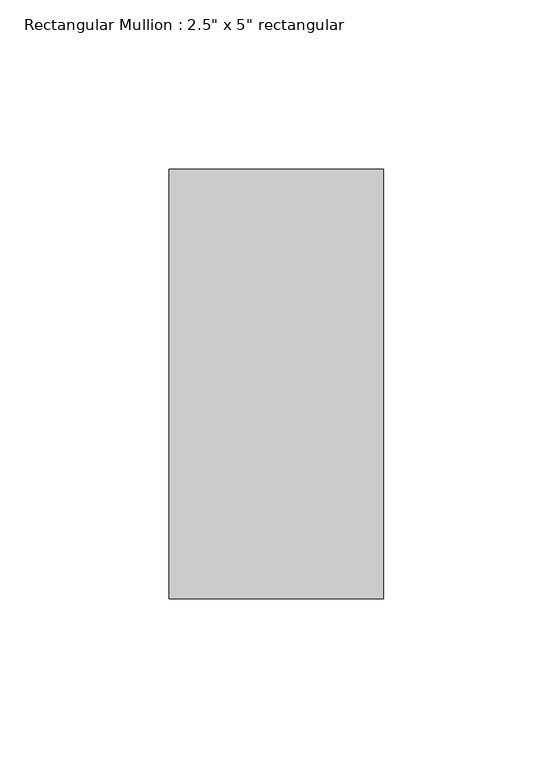
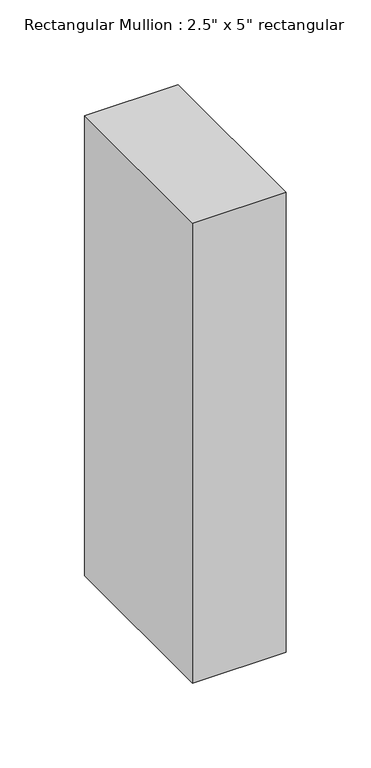
"""IFC4 building model written with IfcOpenShell, lengths in millimetres: member geometry."""

from ifc_helpers import new_model, si_unit, frame, origin, place, context, project, spatial, polyline, outline, extrude, source, transform, mapped, element, save


def member_0c1408be(model_context):
    return source(origin(), model_context, "Body", "SweptSolid", [
        extrude(outline(polyline([(31.75, 63.5), (31.75, -63.5), (-31.75, -63.5), (-31.75, 63.5), (31.75, 63.5)])), frame((0.0, 0.0, -330.2), z_axis=(0.0, 0.0, 1.0), x_axis=(1.0, 0.0, 0.0)), (0.0, 0.0, 1.0), 330.2),
    ])


if __name__ == "__main__":
    model = new_model("IFC4")
    model_context = context("Model", 3, world=origin())
    ifc_project = project(units=[si_unit("LENGTHUNIT", "METRE", prefix="MILLI")], contexts=[model_context])
    site = spatial("IfcSite", under=ifc_project)
    building = spatial("IfcBuilding", under=site)
    placement = place(None, origin())
    member_shape = member_0c1408be(model_context)
    element("IfcMember", 1, ObjectType="Rectangular Mullion : 2.5\" x 5\" rectangular", at=placement, inside=building, context=model_context, shape_type="MappedRepresentation", body=[
        mapped(member_shape, transform((0.0, 0.0, 0.0), x_axis=(1.0, 0.0, 0.0), y_axis=(0.0, 1.0, 0.0), z_axis=(0.0, 0.0, 1.0))),
    ])
    save(model, "model.ifc")

# Revit data of these elements
# Type "Rectangular Mullion : 2.5\" x 5\" rectangular"
#   built-in parameter 1007304 = 0.416667 (stored number, unit not read)
#   built-in parameter 1007301 = 0.104167 (stored number, unit not read)
#   built-in parameter 1007300 = 0.104167 (stored number, unit not read)
# Element 1 (IfcMember, "Rectangular Mullion : 2.5\" x 5\" rectangular")
#   Materials on its faces: "Aluminum"
# Materials
#   "Aluminum": class "Metal", colour RGB 247 247 247, transparency 0, Description = "Aluminum 6061", Cost = 0
